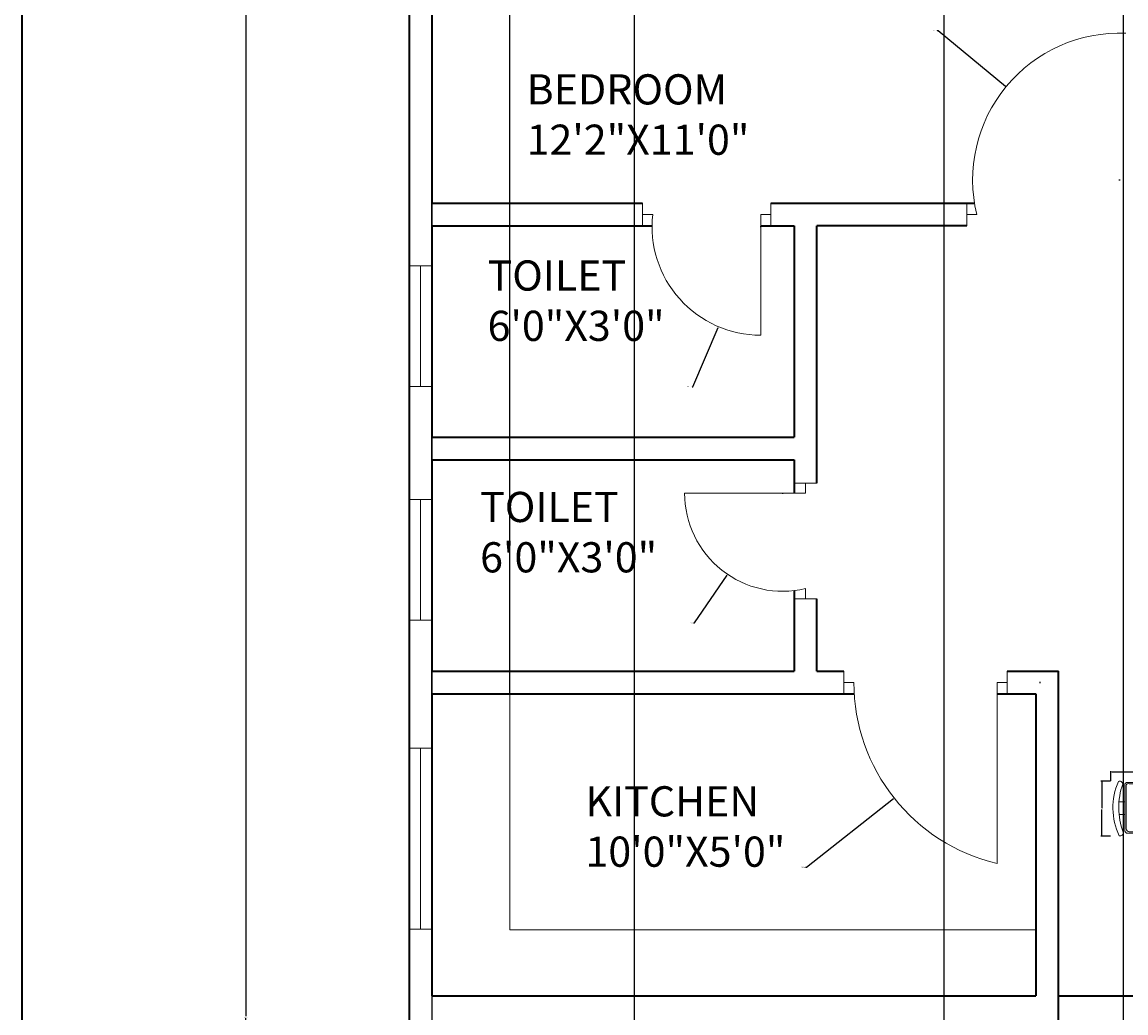
# Model space of a CAD drawing. Units: inches. Extents: x 1721 to 2510, y 1544 to 2360.
# Tile 6 of 10: x 1721 to 1940, y 1988 to 2185. Entities that reach past the tile are written whole.
import ezdxf

# ---------------------------------------------------------------- set-up
doc = ezdxf.new("R2010")
doc.units = ezdxf.units.IN
for name, color, linetype, lineweight in [('A-ANNO-DIMS', 2, 'Continuous', 18), ('A-ANNO-TTLB', 7, 'Continuous', 35), ('A-AREA-IDEN', 7, 'Continuous', 18), ('A-DOOR', 3, 'Continuous', 18), ('A-FLOR-FIXT', 9, 'Continuous', 18), ('A-FURN', 8, 'Continuous', 13), ('A-GLAZ', 4, 'Continuous', 18), ('A-WALL', 7, 'Continuous', 35)]:
    doc.layers.add(name, color=color, linetype=linetype, lineweight=lineweight)
doc.styles.get("Standard").update_dxf_attribs({"font": 'arial.ttf'})
doc.dimstyles.get("Standard").update_dxf_attribs({"dimtxt": 0.18, "dimasz": 0.18, "dimexe": 0.18, "dimexo": 0.0625, "dimgap": 0.09, "dimtad": 0, "dimtih": 1, "dimtoh": 1, "dimdec": 4, "dimzin": 0, "dimdsep": 46, "dimtxsty": 'Standard', "dimcen": 0.09, "dimadec": 0, "dimazin": 0, "dimtfac": 1, "dimtdec": 4, "dimtofl": 0, "dimtmove": 0, "dimatfit": 3, "dimfxl": 1, "dimtolj": 1, "dimtzin": 0, "dimarcsym": 0})

# ---------------------------------------------------------------- blocks, each defined once
blk = doc.blocks.new('WIN-24IN-A')
for p, q in [((4.5, 24), (0, 24)), ((0, 24), (2.25, 24)), ((2.25, 24), (2.25, 0)), ((4.5, 0), (0, 0)), ((2.25, 0), (4.5, 0))]:
    blk.add_line(p, q)
blk = doc.blocks.new('WIN-24IN-B')
for p, q in [((0, 24), (4.5, 24)), ((4.5, 24), (2.25, 24)), ((2.25, 24), (2.25, 0)), ((4.5, 0), (0, 0)), ((2.25, 0), (4.5, 0))]:
    blk.add_line(p, q)
blk = doc.blocks.new('WIN-36IN-B')
for p, q in [((4.5, 36), (0, 36)), ((2.25, 0), (2.25, 36)), ((2.25, 36), (4.5, 36)), ((0, 0), (4.5, 0)), ((4.5, 0), (2.25, 0))]:
    blk.add_line(p, q)
blk = doc.blocks.new('CHAIR-DINING-A')
for points in [[(2.02, 0.75, -0.578392), (1.23, 0.03, -0.214524), (1.08, 10.81, -0.552014), (1.95, 10.31, 0.175809), (2.02, 0.75)], [(2.34, 10.03, -0.414214), (2.96, 10.65), (11.11, 10.65, -0.414214), (11.73, 10.03), (11.73, 1.16, -0.414214), (11.11, 0.54), (2.96, 0.54, -0.414214), (2.34, 1.16), (2.34, 10.03)], [(2.34, 4.27), (1.21, 4.27, 0.064759)]]:
    blk.add_lwpolyline(points, format="xyb")
blk.add_lwpolyline([(2.62, 10.02), (2.62, 1.44, 0.414214), (3.24, 0.82), (10.83, 0.82, 0.414214), (11.45, 1.44), (11.45, 10.02, 0.512069), (10.83, 10.37), (3.24, 10.37, 0.512069)], format="xyb", close=True)
blk.add_lwpolyline([(1.19, 6.76), (2.34, 6.76)])
blk = doc.blocks.new('*D30')
at = {"layer": 'A-ANNO-DIMS', "color": 0, "lineweight": -2, "transparency": 16777216}
for p, q in [((1937.43, 2033.84), (1937.43, 2035.78)), ((1937.61, 2035.6), (1942.43, 2035.6)), ((1949.39, 2035.6), (1944.57, 2035.6)), ((1949.57, 2033.84), (1949.57, 2035.78))]:
    blk.add_line(p, q, dxfattribs=at)
at = {"layer": 'A-ANNO-DIMS', "color": 0, "transparency": 16777216}
for points in [[(1937.61, 2035.63), (1937.61, 2035.57), (1937.43, 2035.6)], [(1949.39, 2035.63), (1949.39, 2035.57), (1949.57, 2035.6)]]:
    blk.add_solid(points, dxfattribs=at)
at = {"layer": 'Defpoints', "color": 0, "transparency": 16777216}
for p in [(1949.57, 2035.6), (1937.43, 2033.78), (1949.57, 2033.78)]:
    blk.add_point(p, dxfattribs=at)
at = {"layer": 'A-ANNO-DIMS', "color": 0, "transparency": 16777216, "insert": (1943.5, 2035.6), "char_height": 0.18, "attachment_point": 5}
blk.add_mtext('\\A1;CHAIR A 12 TYP.', dxfattribs=at)
blk = doc.blocks.new('*D31')
at = {"layer": 'A-ANNO-DIMS', "color": 0, "lineweight": -2, "transparency": 16777216}
for p, q in [((1937.37, 2033.78), (1935.43, 2033.78)), ((1935.61, 2033.6), (1935.61, 2028.49)), ((1935.61, 2023.02), (1935.61, 2028.13)), ((1937.37, 2022.84), (1935.43, 2022.84))]:
    blk.add_line(p, q, dxfattribs=at)
at = {"layer": 'A-ANNO-DIMS', "color": 0, "transparency": 16777216}
for points in [[(1935.58, 2033.6), (1935.64, 2033.6), (1935.61, 2033.78)], [(1935.58, 2023.02), (1935.64, 2023.02), (1935.61, 2022.84)]]:
    blk.add_solid(points, dxfattribs=at)
at = {"layer": 'Defpoints', "color": 0, "transparency": 16777216}
for p in [(1935.61, 2033.78), (1937.43, 2033.78), (1937.43, 2022.84)]:
    blk.add_point(p, dxfattribs=at)
at = {"layer": 'A-ANNO-DIMS', "color": 0, "transparency": 16777216, "insert": (1935.61, 2028.31), "char_height": 0.18, "attachment_point": 5}
blk.add_mtext('\\A1;11 TYP.', dxfattribs=at)
blk = doc.blocks.new('*D41')
at = {"layer": 'A-ANNO-DIMS', "color": 0, "lineweight": -2, "transparency": 16777216}
for p, q in [((1797.94, 2285.13), (1765.42, 2285.13)), ((1765.6, 2284.95), (1765.6, 1987.06)), ((1765.6, 1688.81), (1765.6, 1986.7)), ((1797.94, 1688.63), (1765.42, 1688.63))]:
    blk.add_line(p, q, dxfattribs=at)
at = {"layer": 'A-ANNO-DIMS', "color": 0, "transparency": 16777216}
for points in [[(1765.57, 2284.95), (1765.63, 2284.95), (1765.6, 2285.13)], [(1765.57, 1688.81), (1765.63, 1688.81), (1765.6, 1688.63)]]:
    blk.add_solid(points, dxfattribs=at)
at = {"layer": 'Defpoints', "color": 0, "transparency": 16777216}
for p in [(1765.6, 2285.13), (1798, 2285.13), (1798, 1688.63)]:
    blk.add_point(p, dxfattribs=at)
at = {"layer": 'A-ANNO-DIMS', "color": 0, "transparency": 16777216, "insert": (1765.6, 1986.88), "char_height": 0.18, "attachment_point": 5}
blk.add_mtext('\\A1;596.5', dxfattribs=at)
blk = doc.blocks.new('*D56')
at = {"layer": 'A-ANNO-DIMS', "color": 0, "lineweight": -2, "transparency": 16777216}
for p, q in [((1802.5, 2280.57), (1802.5, 1606.75)), ((1842.73, 2280.57), (1842.73, 1606.75)), ((1802.68, 1606.93), (1822.15, 1606.93)), ((1842.55, 1606.93), (1823.08, 1606.93))]:
    blk.add_line(p, q, dxfattribs=at)
at = {"layer": 'A-ANNO-DIMS', "color": 0, "transparency": 16777216}
for points in [[(1802.68, 1606.96), (1802.68, 1606.9), (1802.5, 1606.93)], [(1842.55, 1606.96), (1842.55, 1606.9), (1842.73, 1606.93)]]:
    blk.add_solid(points, dxfattribs=at)
at = {"layer": 'Defpoints', "color": 0, "transparency": 16777216}
for p in [(1802.5, 2280.63), (1842.73, 2280.63), (1842.73, 1606.93)]:
    blk.add_point(p, dxfattribs=at)
at = {"layer": 'A-ANNO-DIMS', "color": 0, "transparency": 16777216, "insert": (1822.61, 1606.93), "char_height": 0.18, "attachment_point": 5}
blk.add_mtext('\\A1;40.224', dxfattribs=at)
blk = doc.blocks.new('*D59')
at = {"layer": 'A-ANNO-DIMS', "color": 0, "lineweight": -2, "transparency": 16777216}
for p, q in [((1904.34, 1857.19), (1904.34, 2317.71)), ((1904.52, 2317.53), (1921.76, 2317.53)), ((1939.78, 2317.53), (1922.54, 2317.53)), ((1939.96, 1857.19), (1939.96, 2317.71))]:
    blk.add_line(p, q, dxfattribs=at)
at = {"layer": 'A-ANNO-DIMS', "color": 0, "transparency": 16777216}
for points in [[(1904.52, 2317.56), (1904.52, 2317.5), (1904.34, 2317.53)], [(1939.78, 2317.56), (1939.78, 2317.5), (1939.96, 2317.53)]]:
    blk.add_solid(points, dxfattribs=at)
at = {"layer": 'Defpoints', "color": 0, "transparency": 16777216}
for p in [(1939.96, 2317.53), (1904.34, 1857.13), (1939.96, 1857.13)]:
    blk.add_point(p, dxfattribs=at)
at = {"layer": 'A-ANNO-DIMS', "color": 0, "transparency": 16777216, "insert": (1922.15, 2317.53), "char_height": 0.18, "attachment_point": 5}
blk.add_mtext('\\A1;35.62', dxfattribs=at)
blk = doc.blocks.new('*D66')
at = {"layer": 'A-ANNO-DIMS', "color": 0, "lineweight": -2, "transparency": 16777216}
for p, q in [((1802.5, 2051.19), (1802.5, 2317.71)), ((1802.68, 2317.53), (1809.89, 2317.53)), ((1817.87, 2317.53), (1810.66, 2317.53)), ((1818.05, 2051.19), (1818.05, 2317.71))]:
    blk.add_line(p, q, dxfattribs=at)
at = {"layer": 'A-ANNO-DIMS', "color": 0, "transparency": 16777216}
for points in [[(1802.68, 2317.56), (1802.68, 2317.5), (1802.5, 2317.53)], [(1817.87, 2317.56), (1817.87, 2317.5), (1818.05, 2317.53)]]:
    blk.add_solid(points, dxfattribs=at)
at = {"layer": 'Defpoints', "color": 0, "transparency": 16777216}
for p in [(1818.05, 2317.53), (1802.5, 2051.13), (1818.05, 2051.13)]:
    blk.add_point(p, dxfattribs=at)
at = {"layer": 'A-ANNO-DIMS', "color": 0, "transparency": 16777216, "insert": (1810.28, 2317.53), "char_height": 0.18, "attachment_point": 5}
blk.add_mtext('\\A1;15.55', dxfattribs=at)
blk = doc.blocks.new('*D70')
at = {"layer": 'A-ANNO-DIMS', "color": 0, "lineweight": -2, "transparency": 16777216}
for p, q in [((1923.28, 2053.38), (1923.46, 2053.38)), ((1923.37, 2053.29), (1923.37, 2053.47)), ((1876.95, 2016.66), (1894.22, 2030.32)), ((1876.77, 2016.66), (1876.95, 2016.66))]:
    blk.add_line(p, q, dxfattribs=at)
at = {"layer": 'A-ANNO-DIMS', "color": 0, "transparency": 16777216}
blk.add_solid([(1894.2, 2030.34), (1894.23, 2030.29), (1894.36, 2030.43)], dxfattribs=at)
at = {"layer": 'Defpoints', "color": 0, "transparency": 16777216}
for p in [(1923.37, 2053.38), (1894.36, 2030.43)]:
    blk.add_point(p, dxfattribs=at)
at = {"layer": 'A-ANNO-DIMS', "color": 0, "transparency": 16777216, "insert": (1876.29, 2016.66), "char_height": 0.18, "attachment_point": 5}
blk.add_mtext('\\A1;R36.99', dxfattribs=at)
blk = doc.blocks.new('*D78')
at = {"layer": 'A-ANNO-DIMS', "color": 0, "lineweight": -2, "transparency": 16777216}
for p, q in [((1902.92, 2182.9), (1903.1, 2182.9)), ((1903.1, 2182.9), (1916.49, 2171.88)), ((1939.07, 2153.22), (1939.25, 2153.22)), ((1939.16, 2153.13), (1939.16, 2153.31))]:
    blk.add_line(p, q, dxfattribs=at)
at = {"layer": 'A-ANNO-DIMS', "color": 0, "transparency": 16777216}
blk.add_solid([(1916.51, 2171.91), (1916.47, 2171.86), (1916.63, 2171.77)], dxfattribs=at)
at = {"layer": 'Defpoints', "color": 0, "transparency": 16777216}
for p in [(1916.63, 2171.77), (1939.16, 2153.22)]:
    blk.add_point(p, dxfattribs=at)
at = {"layer": 'A-ANNO-DIMS', "color": 0, "transparency": 16777216, "insert": (1902.44, 2182.9), "char_height": 0.18, "attachment_point": 5}
blk.add_mtext('\\A1;R29.19', dxfattribs=at)
blk = doc.blocks.new('*D86')
at = {"layer": 'A-ANNO-DIMS', "color": 0, "lineweight": -2, "transparency": 16777216}
for p, q in [((1867.78, 2143.97), (1867.96, 2143.97)), ((1867.87, 2143.88), (1867.87, 2144.06)), ((1854.41, 2112.15), (1859.39, 2123.92)), ((1854.23, 2112.15), (1854.41, 2112.15))]:
    blk.add_line(p, q, dxfattribs=at)
at = {"layer": 'A-ANNO-DIMS', "color": 0, "transparency": 16777216}
blk.add_solid([(1859.36, 2123.93), (1859.42, 2123.91), (1859.46, 2124.08)], dxfattribs=at)
at = {"layer": 'Defpoints', "color": 0, "transparency": 16777216}
for p in [(1867.87, 2143.97), (1859.46, 2124.08)]:
    blk.add_point(p, dxfattribs=at)
at = {"layer": 'A-ANNO-DIMS', "color": 0, "transparency": 16777216, "insert": (1853.68, 2112.15), "char_height": 0.18, "attachment_point": 5}
blk.add_mtext('\\A1;R21.595', dxfattribs=at)
blk = doc.blocks.new('*D87')
at = {"layer": 'A-ANNO-DIMS', "color": 0, "lineweight": -2, "transparency": 16777216}
for p, q in [((1872.16, 2090.99), (1872.34, 2090.99)), ((1872.25, 2090.9), (1872.25, 2091.08)), ((1854.69, 2065.2), (1861.17, 2074.72)), ((1854.51, 2065.2), (1854.69, 2065.2))]:
    blk.add_line(p, q, dxfattribs=at)
at = {"layer": 'A-ANNO-DIMS', "color": 0, "transparency": 16777216}
blk.add_solid([(1861.15, 2074.74), (1861.2, 2074.71), (1861.28, 2074.87)], dxfattribs=at)
at = {"layer": 'Defpoints', "color": 0, "transparency": 16777216}
for p in [(1872.25, 2090.99), (1861.28, 2074.87)]:
    blk.add_point(p, dxfattribs=at)
at = {"layer": 'A-ANNO-DIMS', "color": 0, "transparency": 16777216, "insert": (1854.1, 2065.2), "char_height": 0.18, "attachment_point": 5}
blk.add_mtext('\\A1;R19.5', dxfattribs=at)

msp = doc.modelspace()

# ---------------------------------------------------------------- linework, layer by layer
at = {"layer": 'A-ANNO-TTLB'}
msp.add_lwpolyline([(1721.1268, 2360.2177), (2509.707, 2360.2177), (2509.707, 1544.3037), (1721.1268, 1544.3037)], close=True, dxfattribs=at)
at = {"layer": 'A-DOOR'}
for p, q in [((1844.4053, 2148.6298), (1844.4053, 2148.6298)), ((1844.4053, 2148.6298), (1844.4053, 2148.6298)), ((1844.4053, 2148.6298), (1844.4053, 2144.1298)), ((1869.8657, 2148.6298), (1869.8657, 2144.1298)), ((1908.7837, 2148.6298), (1908.7837, 2144.1298)), ((1844.4053, 2144.1298), (1844.4053, 2146.3798)), ((1844.4053, 2146.3798), (1846.4053, 2146.3798)), ((1869.8657, 2146.3798), (1867.8657, 2146.3798)), ((1867.8657, 2146.3798), (1867.8657, 2122.3798)), ((1869.8657, 2144.1298), (1869.8657, 2146.3798)), ((1908.7837, 2144.1298), (1908.7837, 2146.3798)), ((1908.7837, 2146.3798), (1910.7837, 2146.3798)), ((1844.4053, 2144.1298), (1844.4053, 2144.1298)), ((1874.5024, 2092.99), (1879.0024, 2092.99)), ((1879.0024, 2092.99), (1876.7524, 2092.99)), ((1876.7524, 2092.99), (1876.7524, 2090.99)), ((1876.7524, 2090.99), (1852.7524, 2090.99)), ((1876.7524, 2070.0182), (1876.7524, 2072.0182)), ((1874.5024, 2070.0182), (1879.0024, 2070.0182)), ((1879.0024, 2070.0182), (1876.7524, 2070.0182)), ((1884.3748, 2055.6298), (1884.3748, 2051.1298)), ((1916.8571, 2055.6298), (1916.8571, 2051.1298)), ((1884.3748, 2051.1298), (1884.3748, 2053.3798)), ((1884.3748, 2053.3798), (1886.3748, 2053.3798)), ((1916.8571, 2053.3798), (1914.8571, 2053.3798)), ((1914.8571, 2053.3798), (1914.8571, 2017.3798)), ((1916.8571, 2051.1298), (1916.8571, 2053.3798))]:
    msp.add_line(p, q, dxfattribs=at)
for centre, radius, start, end in [((1939.163, 2153.2159), 29.191, 87.529641, 193.543609), ((1867.8657, 2143.9746), 21.5947, 173.605045, 270), ((1872.2509, 2090.99), 19.4985, 180, 283.347802), ((1923.367, 2053.3798), 36.9921, 180, 256.700233)]:
    msp.add_arc(centre, radius, start, end, dxfattribs=at)
at = {"layer": 'A-FLOR-FIXT'}
for p, q in [((1818.0518, 2051.1298), (1818.0518, 2004.2331)), ((1818.0518, 2004.2331), (1922.5024, 2004.2331))]:
    msp.add_line(p, q, dxfattribs=at)
at = {"layer": 'A-WALL'}
for p, q in [((1798.0024, 2285.1298), (1798.0024, 1688.6298)), ((1802.5024, 2280.6298), (1802.5024, 2148.6298)), ((1802.5024, 2148.6298), (1844.4053, 2148.6298)), ((1802.5024, 2148.6298), (1844.4053, 2148.6298)), ((1869.8657, 2148.6298), (1874.5024, 2148.6298)), ((1869.8657, 2148.6298), (1879.0024, 2148.6298)), ((1879.0024, 2148.6298), (1910.3345, 2148.6298)), ((1802.5024, 2144.1298), (1846.2715, 2144.1298)), ((1802.5024, 2144.1298), (1802.5024, 2102.1298)), ((1867.8657, 2144.1298), (1874.5024, 2144.1298)), ((1874.5024, 2144.1298), (1874.5024, 2102.1298)), ((1908.7837, 2144.1298), (1879.0024, 2144.1298)), ((1879.0024, 2092.99), (1879.0024, 2144.1298)), ((1802.5024, 2102.1298), (1874.5024, 2102.1298)), ((1802.5024, 2097.6298), (1874.5024, 2097.6298)), ((1802.5024, 2097.6298), (1802.5024, 2055.6298)), ((1874.5024, 2097.6298), (1874.5024, 2090.99)), ((1874.5024, 2071.6219), (1874.5024, 2055.6298)), ((1879.0024, 2055.6298), (1879.0024, 2070.0182)), ((1802.5024, 2055.6298), (1874.5024, 2055.6298)), ((1879.0024, 2055.6298), (1884.3748, 2055.6298)), ((1916.8571, 2055.6298), (1927.0024, 2055.6298)), ((1927.0024, 1922.1298), (1927.0024, 2055.6298)), ((1802.5024, 2051.1298), (1886.4433, 2051.1298)), ((1802.5024, 2051.1298), (1886.4433, 2051.1298)), ((1802.5024, 2051.1298), (1802.5024, 1991.1298)), ((1874.5024, 2051.1298), (1879.0024, 2051.1298)), ((1914.8571, 2051.1298), (1922.5024, 2051.1298)), ((1914.8571, 2051.1298), (1922.5024, 2051.1298)), ((1922.5024, 2051.1298), (1922.5024, 1991.1298)), ((1802.5024, 1991.1298), (1922.5024, 1991.1298)), ((1927.0024, 1991.1298), (2051.9528, 1991.1298))]:
    msp.add_line(p, q, dxfattribs=at)

# ---------------------------------------------------------------- block references
at = {"layer": 'A-FURN'}
msp.add_blockref('CHAIR-DINING-A', (1937.842, 2022.875), dxfattribs=at)
at = {"layer": 'A-GLAZ', "extrusion": (0, 0, -1), "zscale": -1, "rotation": 180}
msp.add_blockref('WIN-24IN-A', (-1798.002, 2136.182), dxfattribs=at)
at = {"layer": 'A-GLAZ', "extrusion": (0, 0, -1), "zscale": -1}
for name, p in [('WIN-24IN-B', (-1802.5028, 2065.7637)), ('WIN-36IN-B', (-1802.5028, 2004.3392))]:
    msp.add_blockref(name, p, dxfattribs=at)

# ---------------------------------------------------------------- texts
at = {"layer": 'A-AREA-IDEN', "char_height": 6, "attachment_point": 1}
for s, width, insert in [('BEDROOM\\P12\'2"X11\'0"', 73.393498, (1821.3589, 2174.2249)), ('TOILET\\P6\'0"X3\'0"', 96.396403, (1813.6032, 2137.2403)), ('TOILET\\P6\'0"X3\'0"', 96.396403, (1812.1244, 2091.2464)), ('KITCHEN\\P10\'0"X5\'0"', 121.574873, (1833.0501, 2032.7562))]:
    msp.add_mtext_dynamic_manual_height_columns(s, width=width, gutter_width=12.5, heights=[0], dxfattribs=dict(at, insert=insert))

# ---------------------------------------------------------------- dimensions: what is measured, and where the dimension line sits
at = {"layer": 'A-ANNO-DIMS'}
for base, p1, p2, override, picture, middle in [((1818.0518, 2317.5298), (1802.5024, 2051.1298), (1818.0518, 2051.1298), {"dimdec": 2, "dimlfac": 1, "dimrnd": 0, "dimzin": 0, "dimdsep": 46, "dimlunit": 2}, '*D66', (1810.2771, 2317.5298)), ((1939.9594, 2317.5298), (1904.3387, 1857.1298), (1939.9594, 1857.1298), {"dimdec": 2, "dimlfac": 1, "dimrnd": 0, "dimzin": 0, "dimdsep": 46, "dimlunit": 2}, '*D59', (1922.149, 2317.5298)), ((1842.7265, 1606.9297), (1802.5024, 2280.6298), (1842.7265, 2280.6298), {"dimdec": 3, "dimlfac": 1, "dimrnd": 0, "dimzin": 0, "dimdsep": 46, "dimlunit": 2}, '*D56', (1822.6145, 1606.9297))]:
    dim = msp.add_linear_dim(base=base, p1=p1, p2=p2, dimstyle='Standard', override=override, dxfattribs=at)
    dim.commit()
    dim.dimension.update_dxf_attribs({"geometry": picture, "text_midpoint": middle})
dim = msp.add_linear_dim(base=(1765.6024, 2285.1298), p1=(1798.0024, 1688.6298), p2=(1798.0024, 2285.1298), angle=90, dimstyle='Standard', override={"dimdec": 1, "dimlfac": 1, "dimrnd": 0, "dimzin": 0, "dimdsep": 46, "dimlunit": 2}, dxfattribs=at)
dim.commit()
dim.dimension.update_dxf_attribs({"geometry": '*D41', "text_midpoint": (1765.6024, 1986.8798)})
for center, mpoint, override, picture, middle in [((1939.163, 2153.2159), (1916.6266, 2171.7693), {"dimdec": 2, "dimlfac": 1, "dimrnd": 0, "dimzin": 0, "dimdsep": 46, "dimlunit": 2}, '*D78', (1902.4448, 2182.9013)), ((1867.8657, 2143.9746), (1859.4581, 2124.0837), {"dimdec": 3, "dimlfac": 1, "dimrnd": 0, "dimzin": 0, "dimdsep": 46, "dimlunit": 2}, '*D86', (1853.6831, 2112.1492)), ((1872.2509, 2090.99), (1861.2759, 2074.8736), {"dimdec": 1, "dimlfac": 1, "dimrnd": 0, "dimzin": 0, "dimdsep": 46, "dimlunit": 2}, '*D87', (1854.1002, 2065.2037)), ((1923.367, 2053.3798), (1894.3565, 2030.4274), {"dimdec": 2, "dimlfac": 1, "dimrnd": 0, "dimzin": 0, "dimdsep": 46, "dimlunit": 2}, '*D70', (1876.2902, 2016.656))]:
    dim = msp.add_radius_dim(center=center, mpoint=mpoint, dimstyle='Standard', override=override, dxfattribs=at)
    dim.commit()
    dim.dimension.update_dxf_attribs({"geometry": picture, "text_midpoint": middle, "dimtype": 164})
dim = msp.add_linear_dim(base=(1949.5732, 2035.6028), p1=(1937.4302, 2033.7813), p2=(1949.5732, 2033.7813), text='CHAIR A <> TYP.', dimstyle='Standard', override={"dimdec": 0, "dimlfac": 1, "dimrnd": 0, "dimzin": 0, "dimdsep": 46, "dimlunit": 2}, dxfattribs=at)
dim.commit()
dim.dimension.update_dxf_attribs({"geometry": '*D30', "text_midpoint": (1943.5017, 2035.6028)})
dim = msp.add_linear_dim(base=(1935.6087, 2033.7813), p1=(1937.4302, 2022.836), p2=(1937.4302, 2033.7813), angle=90, text='<> TYP.', dimstyle='Standard', override={"dimdec": 0, "dimlfac": 1, "dimrnd": 0, "dimzin": 0, "dimdsep": 46, "dimlunit": 2}, dxfattribs=at)
dim.commit()
dim.dimension.update_dxf_attribs({"geometry": '*D31', "text_midpoint": (1935.6087, 2028.3086)})

doc.saveas('drawing.dxf')
